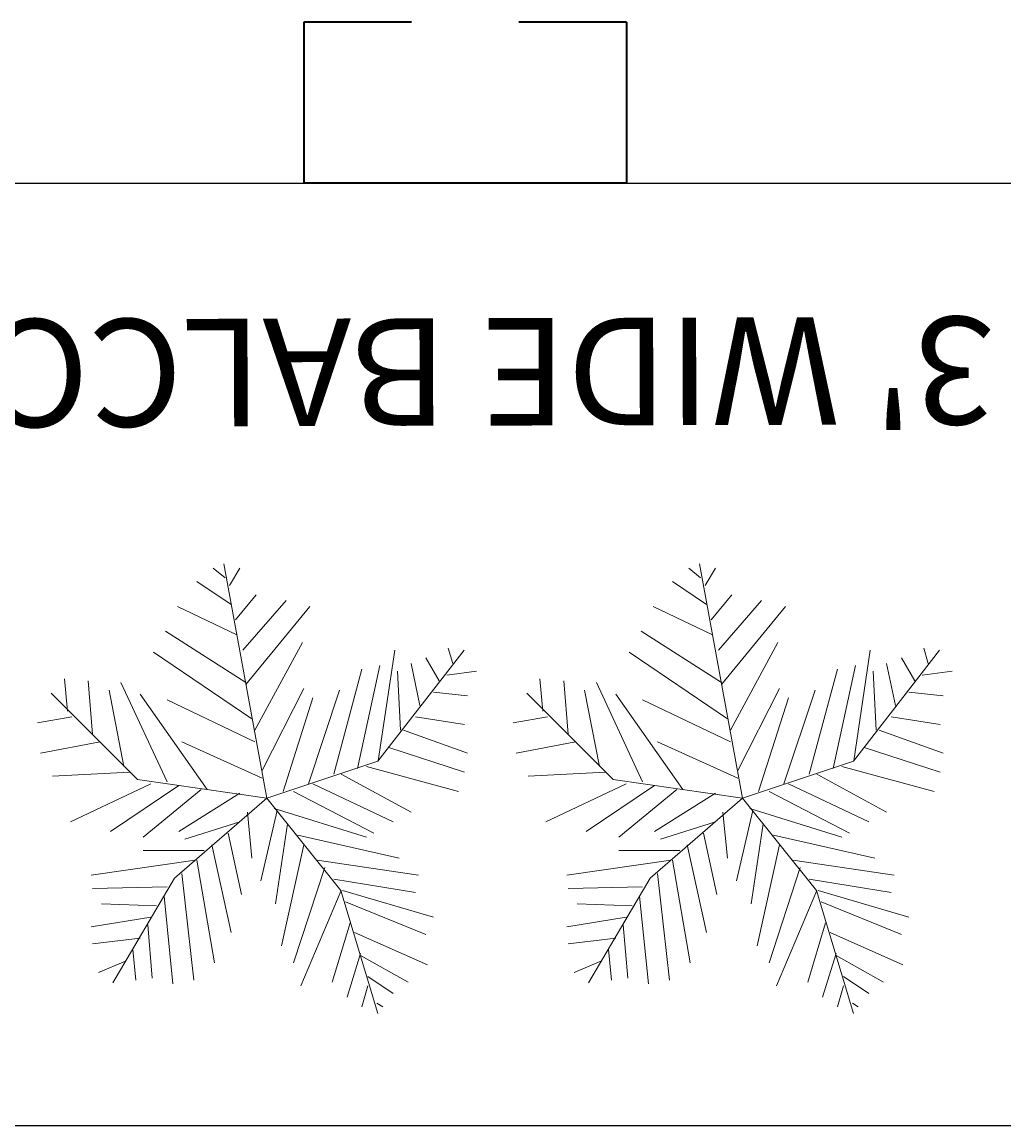
# Model space of a CAD drawing. Units: inches. Extents: x 4159 to 4826, y 299 to 1026.
# Tile 4 of 37: x 4300 to 4354, y 340 to 401. Entities that reach past the tile are written whole.
import ezdxf

# ---------------------------------------------------------------- set-up
doc = ezdxf.new("R2010")
doc.units = ezdxf.units.IN
for name, color, linetype, lineweight in [('A-ANNO-DIMS', 2, 'Continuous', 18), ('A-AREA-IDEN', 7, 'Continuous', 18), ('A-FLOR-BALC', 7, 'Continuous', 25), ('A-WALL', 7, 'Continuous', 35), ('L-PLNT', 94, 'Continuous', 13)]:
    doc.layers.add(name, color=color, linetype=linetype, lineweight=lineweight)
doc.styles.get("Standard").update_dxf_attribs({"font": 'arial.ttf'})
doc.dimstyles.get("Standard").update_dxf_attribs({"dimtxt": 0.18, "dimasz": 0.18, "dimexe": 0.18, "dimexo": 0.0625, "dimgap": 0.09, "dimtad": 0, "dimtih": 1, "dimtoh": 1, "dimdec": 4, "dimzin": 0, "dimdsep": 46, "dimtxsty": 'Standard', "dimcen": 0.09, "dimadec": 0, "dimazin": 0, "dimtfac": 1, "dimtdec": 4, "dimtofl": 0, "dimtmove": 0, "dimatfit": 3, "dimfxl": 1, "dimtolj": 1, "dimtzin": 0, "dimarcsym": 0})

# ---------------------------------------------------------------- blocks, each defined once
blk = doc.blocks.new('*U12')
for p, q in [((0, 0), (-10.5, 57)), ((-10.186, 53.64), (-13.084, 55.962)), ((-9.099, 51.782), (-6.563, 55.962)), ((-8.737, 47.138), (-17.069, 52.711)), ((-7.65, 43.423), (-2.578, 49.46)), ((-7.288, 39.707), (-21.778, 46.673)), ((-5.839, 35.992), (4.667, 48.067)), ((-5.114, 27.632), (10.463, 46.673)), ((-5.114, 28.097), (-24.676, 40.636)), ((-2.941, 16.486), (8.652, 37.85)), ((-3.665, 19.273), (-27.574, 35.527)), ((27, 9), (48, 36)), ((27.127, 9.056), (31.112, 35.992)), ((44.153, 36.456), (45.239, 32.741)), ((22.055, 7.198), (27.489, 32.277)), ((35.096, 32.741), (37.27, 22.524)), ((38.719, 34.134), (41.979, 28.561)), ((16.259, 5.805), (23.142, 31.348)), ((31.836, 30.883), (32.561, 16.486)), ((43.791, 29.954), (51.036, 30.883)), ((-48.585, 21.131), (-49.309, 29.026)), ((-43.513, 28.561), (-42.427, 15.558)), ((-35.544, 28.097), (-24.314, 3.947)), ((-31.5, 4.5), (-52.5, 25.5)), ((-38.442, 26.239), (-34.819, 7.663)), ((-14.533, 2.09), (-30.834, 25.31)), ((-1.129, 6.734), (9.014, 26.704)), ((3.942, 1.625), (11.187, 24.381)), ((10.101, 3.483), (17.708, 26.239)), ((40.53, 25.775), (48.862, 24.846)), ((-24.314, 23.917), (-2.941, 13.7)), ((-47.498, 19.737), (-55.83, 18.344)), ((36.183, 19.737), (48.137, 17.88)), ((33.285, 16.486), (48.862, 10.913)), ((-40.615, 13.7), (-55.105, 10.913)), ((-20.691, 13.7), (-1.129, 4.876)), ((29.662, 12.307), (48.137, 6.269)), ((0, 0), (27, 9)), ((-33.37, 6.269), (-52.207, 5.34)), ((18.07, 5.805), (35.096, -3.483)), ((24.229, 7.663), (46.688, 1.625)), ((-28.299, 3.483), (-47.86, -5.805)), ((-21.416, 3.018), (-38.079, -8.128)), ((0, 0), (-31.5, 4.5)), ((11.187, 3.483), (30.749, -5.805)), ((-15.982, 2.09), (-30.11, -9.521)), ((0, 0), (-22.5, -19.5)), ((-6.563, 1.161), (-21.416, -8.128)), ((0, 0), (18, -22.5)), ((6.478, 1.625), (26.04, -8.592)), ((1.769, -2.555), (24.229, -9.521)), ((-4.752, -3.483), (-3.665, -14.629)), ((2.493, -3.019), (-1.491, -20.202)), ((-6.563, -5.805), (-19.967, -9.985)), ((5.029, -6.27), (2.131, -25.775)), ((-9.461, -8.592), (-6.201, -23.453)), ((7.565, -9.056), (32.198, -14.629)), ((-15.257, -12.772), (-30.11, -12.772)), ((-13.446, -11.378), (-8.737, -32.741)), ((9.014, -11.378), (3.58, -35.992)), ((-17.431, -15.094), (-42.789, -18.809)), ((-17.069, -15.094), (-12.721, -40.172)), ((12.274, -15.094), (36.907, -18.809)), ((-20.691, -18.345), (-17.793, -44.352)), ((14.085, -16.951), (6.478, -40.172)), ((-22.5, -19.5), (-37.5, -45)), ((16.259, -19.738), (36.183, -22.989)), ((-24.314, -21.596), (-42.427, -22.06)), ((-25.038, -23.918), (-22.865, -45.281)), ((18.07, -22.524), (8.289, -45.745)), ((18, -22.5), (27, -52.5)), ((18.433, -22.524), (40.53, -29.026)), ((-26.849, -26.24), (-40.253, -25.775)), ((19.157, -25.311), (38.719, -33.206)), ((-28.299, -29.026), (-42.789, -31.348)), ((-29.023, -30.884), (-27.936, -43.887)), ((20.244, -30.419), (15.897, -44.816)), ((-30.834, -34.135), (-42.427, -35.528)), ((21.331, -32.741), (39.081, -40.636)), ((-32.646, -36.921), (-31.921, -44.352)), ((-34.457, -39.708), (-40.978, -42.494)), ((22.78, -37.85), (19.519, -48.532)), ((22.78, -38.314), (34.372, -44.816)), ((24.591, -43.423), (30.749, -47.603)), ((24.591, -45.745), (23.142, -50.854)), ((26.764, -49.925), (28.213, -50.854))]:
    blk.add_line(p, q)
blk = doc.blocks.new('*D44')
at = {"layer": 'A-ANNO-DIMS', "color": 0, "lineweight": -2, "transparency": 16777216}
for p, q in [((4287.263, 963.093), (4158.88, 963.093)), ((4159.06, 962.913), (4159.06, 647.826)), ((4159.06, 332.375), (4159.06, 647.462)), ((4447.248, 332.195), (4158.88, 332.195))]:
    blk.add_line(p, q, dxfattribs=at)
at = {"layer": 'A-ANNO-DIMS', "color": 0, "transparency": 16777216}
for points in [[(4159.03, 962.913), (4159.09, 962.913), (4159.06, 963.093)], [(4159.03, 332.375), (4159.09, 332.375), (4159.06, 332.195)]]:
    blk.add_solid(points, dxfattribs=at)
at = {"layer": 'Defpoints', "color": 0, "transparency": 16777216}
for p in [(4287.326, 963.093), (4159.06, 332.195), (4447.31, 332.195)]:
    blk.add_point(p, dxfattribs=at)
at = {"layer": 'A-ANNO-DIMS', "color": 0, "transparency": 16777216, "insert": (4159.06, 647.644), "char_height": 0.18, "attachment_point": 5}
blk.add_mtext('\\A1;630.9', dxfattribs=at)
blk = doc.blocks.new('*D46')
at = {"layer": 'A-ANNO-DIMS', "color": 0, "lineweight": -2, "transparency": 16777216}
for p, q in [((4192.31, 392.192), (4192.31, 298.765)), ((4447.31, 332.133), (4447.31, 298.765)), ((4192.49, 298.945), (4319.519, 298.945)), ((4447.13, 298.945), (4320.101, 298.945))]:
    blk.add_line(p, q, dxfattribs=at)
at = {"layer": 'A-ANNO-DIMS', "color": 0, "transparency": 16777216}
for points in [[(4192.49, 298.975), (4192.49, 298.915), (4192.31, 298.945)], [(4447.13, 298.975), (4447.13, 298.915), (4447.31, 298.945)]]:
    blk.add_solid(points, dxfattribs=at)
at = {"layer": 'Defpoints', "color": 0, "transparency": 16777216}
for p in [(4192.31, 392.254), (4447.31, 332.195), (4447.31, 298.945)]:
    blk.add_point(p, dxfattribs=at)
at = {"layer": 'A-ANNO-DIMS', "color": 0, "transparency": 16777216, "insert": (4319.81, 298.945), "char_height": 0.18, "attachment_point": 5}
blk.add_mtext('\\A1;255', dxfattribs=at)

msp = doc.modelspace()

# ---------------------------------------------------------------- linework, layer by layer
at = {"layer": 'A-FLOR-BALC'}
msp.add_lwpolyline([(4267.89, 392.254), (4383.821, 392.254), (4383.821, 339.644), (4267.89, 339.644)], close=True, dxfattribs=at)
at = {"layer": 'A-WALL'}
for p, q in [((4321.31, 401.254), (4315.31, 401.254)), ((4315.31, 401.254), (4315.31, 392.254)), ((4333.31, 401.254), (4327.31, 401.254)), ((4333.31, 401.254), (4333.31, 392.254)), ((4333.31, 392.254), (4315.31, 392.254))]:
    msp.add_line(p, q, dxfattribs=at)

# ---------------------------------------------------------------- block references
at = {"layer": 'L-PLNT', "xscale": 0.2292012274639507, "yscale": 0.2292012274639507, "zscale": 0.2292012274639507}
for p in [(4313.241, 357.945), (4339.782, 357.945)]:
    msp.add_blockref('*U12', p, dxfattribs=at)

# ---------------------------------------------------------------- texts
at = {"layer": 'A-AREA-IDEN'}
msp.add_text("3' WIDE BALCONY", height=6, rotation=180.15208, dxfattribs=at).set_placement((4353.858, 384.806))

# ---------------------------------------------------------------- dimensions: what is measured, and where the dimension line sits
at = {"layer": 'A-ANNO-DIMS'}
dim = msp.add_linear_dim(base=(4159.06, 332.195), p1=(4287.326, 963.093), p2=(4447.31, 332.195), angle=90, dimstyle='Standard', override={"dimdec": 1, "dimlfac": 1, "dimrnd": 0, "dimzin": 0, "dimdsep": 46, "dimlunit": 2}, dxfattribs=at)
dim.commit()
dim.dimension.update_dxf_attribs({"geometry": '*D44', "text_midpoint": (4159.06, 647.644)})
dim = msp.add_linear_dim(base=(4447.31, 298.945), p1=(4192.31, 392.254), p2=(4447.31, 332.195), dimstyle='Standard', override={"dimdec": 0, "dimlfac": 1, "dimrnd": 0, "dimzin": 0, "dimdsep": 46, "dimlunit": 2}, dxfattribs=at)
dim.commit()
dim.dimension.update_dxf_attribs({"geometry": '*D46', "text_midpoint": (4319.81, 298.945)})

doc.saveas('drawing.dxf')
